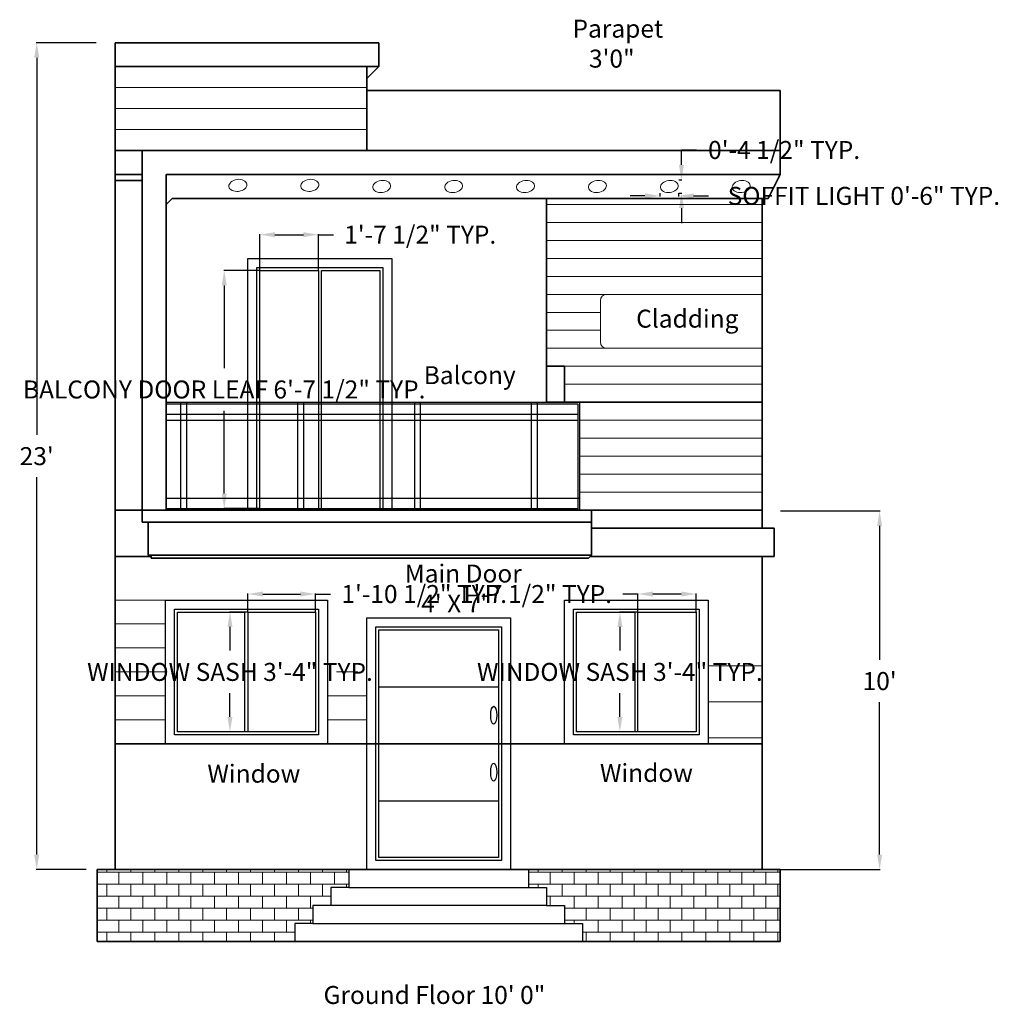
# Model space of a CAD drawing. Units: inches. Extents: x 103 to 430, y 16 to 345.
import ezdxf

# ---------------------------------------------------------------- set-up
doc = ezdxf.new("R2010")
doc.units = ezdxf.units.IN
doc.header["$MEASUREMENT"] = 0
for name, color, linetype, lineweight in [('A-ANNO-DIMS', 2, 'Continuous', 18), ('A-ANNO-TEXT', 7, 'Continuous', 25), ('A-DOOR', 4, 'Continuous', 25), ('A-ELEV', 7, 'Continuous', 35), ('A-ELEV-PATT', 8, 'Continuous', 13), ('A-FLOR-HRAL', 3, 'Continuous', 25), ('A-FLOR-STRS', 3, 'Continuous', 25), ('A-GLAZ', 4, 'Continuous', 25), ('E-LITE', 6, 'Continuous', 18)]:
    doc.layers.add(name, color=color, linetype=linetype, lineweight=lineweight)
doc.styles.get("Standard").update_dxf_attribs({"font": 'arial.ttf'})
doc.dimstyles.get("Standard").update_dxf_attribs({"dimtxt": 6, "dimasz": 5, "dimexe": 0.18, "dimexo": 0.0625, "dimgap": 4, "dimtad": 0, "dimtih": 1, "dimtoh": 1, "dimdec": 0, "dimzin": 0, "dimdsep": 46, "dimlunit": 3, "dimtxsty": 'Standard', "dimcen": 3, "dimadec": 0, "dimazin": 0, "dimtfac": 1, "dimtdec": 0, "dimtofl": 0, "dimtmove": 0, "dimatfit": 3, "dimfxl": 1, "dimtolj": 1, "dimtzin": 0, "dimarcsym": 0})

# ---------------------------------------------------------------- blocks, each defined once
blk = doc.blocks.new('*D1')
at = {"layer": 'A-ANNO-DIMS', "color": 0, "lineweight": -2, "transparency": 16777216}
for p, q in [((128.46, 336.91), (108.43, 336.91)), ((108.61, 331.91), (108.61, 205.97)), ((108.61, 65.91), (108.61, 191.84)), ((125.06, 60.91), (108.43, 60.91))]:
    blk.add_line(p, q, dxfattribs=at)
at = {"layer": 'A-ANNO-DIMS', "color": 0, "transparency": 16777216}
for points in [[(107.77, 331.91), (109.44, 331.91), (108.61, 336.91)], [(107.77, 65.91), (109.44, 65.91), (108.61, 60.91)]]:
    blk.add_solid(points, dxfattribs=at)
at = {"layer": 'Defpoints', "color": 0, "transparency": 16777216}
for p in [(128.53, 336.91), (108.61, 60.91), (125.12, 60.91)]:
    blk.add_point(p, dxfattribs=at)
at = {"layer": 'A-ANNO-DIMS', "color": 0, "transparency": 16777216, "insert": (108.61, 198.91), "char_height": 6, "attachment_point": 5}
blk.add_mtext("\\A1;23'", dxfattribs=at)
blk = doc.blocks.new('*D2')
at = {"layer": 'A-ANNO-DIMS', "color": 0, "lineweight": -2, "transparency": 16777216}
for p, q in [((356.83, 180.64), (390.15, 180.64)), ((389.97, 175.64), (389.97, 130.9)), ((389.97, 65.91), (389.97, 116.77)), ((356.83, 60.91), (390.15, 60.91))]:
    blk.add_line(p, q, dxfattribs=at)
at = {"layer": 'A-ANNO-DIMS', "color": 0, "transparency": 16777216}
for points in [[(389.14, 175.64), (390.8, 175.64), (389.97, 180.64)], [(389.14, 65.91), (390.8, 65.91), (389.97, 60.91)]]:
    blk.add_solid(points, dxfattribs=at)
at = {"layer": 'Defpoints', "color": 0, "transparency": 16777216}
for p in [(356.77, 180.64), (389.97, 180.64), (356.77, 60.91)]:
    blk.add_point(p, dxfattribs=at)
at = {"layer": 'A-ANNO-DIMS', "color": 0, "transparency": 16777216, "insert": (389.97, 123.84), "char_height": 6, "attachment_point": 5}
blk.add_mtext("\\A1;10'", dxfattribs=at)
blk = doc.blocks.new('DOOR-LEAF-BALC')
for p, q in [((0, 79.5), (19.5, 79.5)), ((0, 0), (0, 79.5)), ((19.5, 79.5), (19.5, 0))]:
    blk.add_line(p, q)
blk = doc.blocks.new('WIN-SASH-540')
blk.add_line((0, 40), (0, 0))
blk.add_lwpolyline([(0, 40), (22.5, 40), (22.5, 0), (0, 0)])
blk = doc.blocks.new('WIN-SASH-480')
blk.add_line((19.5, 40), (19.5, 0))
blk.add_lwpolyline([(19.5, 0), (0, 0), (0, 40), (19.5, 40)])
blk = doc.blocks.new('SOFFIT-LIGHT')
blk.add_ellipse((2.99, 2.02), major_axis=(2.98, 0.38), ratio=0.666667)
blk = doc.blocks.new('*D7')
at = {"layer": 'A-ANNO-DIMS', "color": 0, "lineweight": -2, "transparency": 16777216}
for p, q in [((316.65, 286.65), (316.65, 285.6)), ((322.88, 286.65), (322.88, 285.6)), ((311.65, 285.78), (306.65, 285.78)), ((327.88, 285.78), (332.88, 285.78))]:
    blk.add_line(p, q, dxfattribs=at)
at = {"layer": 'A-ANNO-DIMS', "color": 0, "transparency": 16777216}
for points in [[(311.65, 286.61), (311.65, 284.95), (316.65, 285.78)], [(327.88, 286.61), (327.88, 284.95), (322.88, 285.78)]]:
    blk.add_solid(points, dxfattribs=at)
at = {"layer": 'Defpoints', "color": 0, "transparency": 16777216}
for p in [(316.65, 286.71), (322.88, 286.71), (322.88, 285.78)]:
    blk.add_point(p, dxfattribs=at)
at = {"layer": 'A-ANNO-DIMS', "color": 0, "transparency": 16777216, "insert": (384.72, 285.78), "char_height": 6, "attachment_point": 5}
blk.add_mtext('\\A1;SOFFIT LIGHT 0\'-6" TYP.', dxfattribs=at)
blk = doc.blocks.new('*D8')
at = {"layer": 'A-ANNO-DIMS', "color": 0, "lineweight": -2, "transparency": 16777216}
for p, q in [((323.82, 296.1), (323.82, 301.1)), ((323.82, 301.1), (328.82, 301.1)), ((322.94, 291.1), (324, 291.1)), ((322.94, 286.71), (324, 286.71)), ((323.82, 281.71), (323.82, 276.71))]:
    blk.add_line(p, q, dxfattribs=at)
at = {"layer": 'A-ANNO-DIMS', "color": 0, "transparency": 16777216}
for points in [[(322.98, 296.1), (324.65, 296.1), (323.82, 291.1)], [(322.98, 281.71), (324.65, 281.71), (323.82, 286.71)]]:
    blk.add_solid(points, dxfattribs=at)
at = {"layer": 'Defpoints', "color": 0, "transparency": 16777216}
for p in [(322.88, 291.1), (323.82, 291.1), (322.88, 286.71)]:
    blk.add_point(p, dxfattribs=at)
at = {"layer": 'A-ANNO-DIMS', "color": 0, "transparency": 16777216, "insert": (358.09, 301.1), "char_height": 6, "attachment_point": 5}
blk.add_mtext('\\A1;0\'-4 1/2" TYP.', dxfattribs=at)
blk = doc.blocks.new('*D9')
at = {"layer": 'A-ANNO-DIMS', "color": 0, "lineweight": -2, "transparency": 16777216}
for p, q in [((183.06, 260.91), (171.02, 260.91)), ((171.2, 255.91), (171.2, 228.26)), ((171.2, 186.41), (171.2, 214.05)), ((183.06, 181.41), (171.02, 181.41))]:
    blk.add_line(p, q, dxfattribs=at)
at = {"layer": 'A-ANNO-DIMS', "color": 0, "transparency": 16777216}
for points in [[(170.36, 255.91), (172.03, 255.91), (171.2, 260.91)], [(170.36, 186.41), (172.03, 186.41), (171.2, 181.41)]]:
    blk.add_solid(points, dxfattribs=at)
at = {"layer": 'Defpoints', "color": 0, "transparency": 16777216}
for p in [(171.2, 260.91), (183.12, 260.91), (183.12, 181.41)]:
    blk.add_point(p, dxfattribs=at)
at = {"layer": 'A-ANNO-DIMS', "color": 0, "transparency": 16777216, "insert": (171.2, 221.16), "char_height": 6, "attachment_point": 5}
blk.add_mtext('\\A1;BALCONY DOOR LEAF 6\'-7 1/2" TYP.', dxfattribs=at)
blk = doc.blocks.new('*D10')
at = {"layer": 'A-ANNO-DIMS', "color": 0, "lineweight": -2, "transparency": 16777216}
for p, q in [((183.12, 260.97), (183.12, 273.01)), ((188.12, 272.83), (197.62, 272.83)), ((202.62, 260.97), (202.62, 273.01)), ((202.62, 272.83), (207.62, 272.83))]:
    blk.add_line(p, q, dxfattribs=at)
at = {"layer": 'A-ANNO-DIMS', "color": 0, "transparency": 16777216}
for points in [[(188.12, 273.66), (188.12, 272), (183.12, 272.83)], [(197.62, 273.66), (197.62, 272), (202.62, 272.83)]]:
    blk.add_solid(points, dxfattribs=at)
at = {"layer": 'Defpoints', "color": 0, "transparency": 16777216}
for p in [(202.62, 272.83), (183.12, 260.91), (202.62, 260.91)]:
    blk.add_point(p, dxfattribs=at)
at = {"layer": 'A-ANNO-DIMS', "color": 0, "transparency": 16777216, "insert": (236.62, 272.83), "char_height": 6, "attachment_point": 5}
blk.add_mtext('\\A1;1\'-7 1/2" TYP.', dxfattribs=at)
blk = doc.blocks.new('*D11')
at = {"layer": 'A-ANNO-DIMS', "color": 0, "lineweight": -2, "transparency": 16777216}
for p, q in [((179.06, 146.89), (172.94, 146.89)), ((173.12, 141.89), (173.12, 134)), ((173.12, 111.89), (173.12, 119.79)), ((179.06, 106.89), (172.94, 106.89))]:
    blk.add_line(p, q, dxfattribs=at)
at = {"layer": 'A-ANNO-DIMS', "color": 0, "transparency": 16777216}
for points in [[(172.29, 141.89), (173.96, 141.89), (173.12, 146.89)], [(172.29, 111.89), (173.96, 111.89), (173.12, 106.89)]]:
    blk.add_solid(points, dxfattribs=at)
at = {"layer": 'Defpoints', "color": 0, "transparency": 16777216}
for p in [(173.12, 146.89), (179.12, 146.89), (179.12, 106.89)]:
    blk.add_point(p, dxfattribs=at)
at = {"layer": 'A-ANNO-DIMS', "color": 0, "transparency": 16777216, "insert": (173.12, 126.89), "char_height": 6, "attachment_point": 5}
blk.add_mtext('\\A1;WINDOW SASH 3\'-4" TYP.', dxfattribs=at)
blk = doc.blocks.new('*D12')
at = {"layer": 'A-ANNO-DIMS', "color": 0, "lineweight": -2, "transparency": 16777216}
for p, q in [((179.12, 146.96), (179.12, 153.07)), ((184.12, 152.89), (196.62, 152.89)), ((201.62, 146.96), (201.62, 153.07)), ((201.62, 152.89), (206.62, 152.89))]:
    blk.add_line(p, q, dxfattribs=at)
at = {"layer": 'A-ANNO-DIMS', "color": 0, "transparency": 16777216}
for points in [[(184.12, 153.73), (184.12, 152.06), (179.12, 152.89)], [(196.62, 153.73), (196.62, 152.06), (201.62, 152.89)]]:
    blk.add_solid(points, dxfattribs=at)
at = {"layer": 'Defpoints', "color": 0, "transparency": 16777216}
for p in [(201.62, 152.89), (179.12, 146.89), (201.62, 146.89)]:
    blk.add_point(p, dxfattribs=at)
at = {"layer": 'A-ANNO-DIMS', "color": 0, "transparency": 16777216, "insert": (237.95, 152.89), "char_height": 6, "attachment_point": 5}
blk.add_mtext('\\A1;1\'-10 1/2" TYP.', dxfattribs=at)
blk = doc.blocks.new('*D13')
at = {"layer": 'A-ANNO-DIMS', "color": 0, "lineweight": -2, "transparency": 16777216}
for p, q in [((309.2, 146.89), (303.09, 146.89)), ((303.27, 141.89), (303.27, 134)), ((303.27, 111.89), (303.27, 119.79)), ((309.2, 106.89), (303.09, 106.89))]:
    blk.add_line(p, q, dxfattribs=at)
at = {"layer": 'A-ANNO-DIMS', "color": 0, "transparency": 16777216}
for points in [[(302.43, 141.89), (304.1, 141.89), (303.27, 146.89)], [(302.43, 111.89), (304.1, 111.89), (303.27, 106.89)]]:
    blk.add_solid(points, dxfattribs=at)
at = {"layer": 'Defpoints', "color": 0, "transparency": 16777216}
for p in [(309.27, 146.89), (303.27, 106.89), (309.27, 106.89)]:
    blk.add_point(p, dxfattribs=at)
at = {"layer": 'A-ANNO-DIMS', "color": 0, "transparency": 16777216, "insert": (303.27, 126.89), "char_height": 6, "attachment_point": 5}
blk.add_mtext('\\A1;WINDOW SASH 3\'-4" TYP.', dxfattribs=at)
blk = doc.blocks.new('*D14')
at = {"layer": 'A-ANNO-DIMS', "color": 0, "lineweight": -2, "transparency": 16777216}
for p, q in [((309.27, 152.89), (304.27, 152.89)), ((309.27, 146.96), (309.27, 153.07)), ((323.77, 152.89), (314.27, 152.89)), ((328.77, 146.96), (328.77, 153.07))]:
    blk.add_line(p, q, dxfattribs=at)
at = {"layer": 'A-ANNO-DIMS', "color": 0, "transparency": 16777216}
for points in [[(314.27, 153.73), (314.27, 152.06), (309.27, 152.89)], [(323.77, 153.73), (323.77, 152.06), (328.77, 152.89)]]:
    blk.add_solid(points, dxfattribs=at)
at = {"layer": 'Defpoints', "color": 0, "transparency": 16777216}
for p in [(309.27, 152.89), (309.27, 146.89), (328.77, 146.89)]:
    blk.add_point(p, dxfattribs=at)
at = {"layer": 'A-ANNO-DIMS', "color": 0, "transparency": 16777216, "insert": (275.27, 152.89), "char_height": 6, "attachment_point": 5}
blk.add_mtext('\\A1;1\'-7 1/2" TYP.', dxfattribs=at)

msp = doc.modelspace()

# ---------------------------------------------------------------- hatches: boundary and pattern name
at = {"layer": 'A-ELEV-PATT'}
h = msp.add_hatch(dxfattribs=at)
h.set_pattern_fill('AR-B816', color=256, scale=0.5)
h.paths.add_polyline_path([(206.77, 54.91), (212.77, 54.91), (212.77, 60.91), (134.77, 60.91), (128.77, 60.91), (128.77, 36.91), (134.77, 36.91), (194.77, 36.91), (194.77, 42.91), (200.77, 42.91), (200.77, 48.91), (206.77, 48.91)])
h.paths.add_polyline_path([(356.77, 60.91), (350.77, 60.91), (272.77, 60.91), (272.77, 54.91), (278.77, 54.91), (278.77, 48.91), (284.77, 48.91), (284.77, 42.91), (290.77, 42.91), (290.77, 36.91), (350.77, 36.91), (356.77, 36.91)])

# ---------------------------------------------------------------- linework, layer by layer
at = {"layer": 'A-DOOR'}
for p, q in [((179.12, 181.41), (179.12, 264.91)), ((179.12, 264.91), (227.12, 264.91)), ((227.12, 264.91), (227.12, 181.41)), ((182.12, 181.41), (182.12, 261.91)), ((182.12, 261.91), (224.12, 261.91)), ((224.12, 261.91), (224.12, 181.41)), ((222.77, 121.91), (262.77, 121.91)), ((222.77, 102.91), (262.77, 102.91)), ((222.77, 83.91), (262.77, 83.91))]:
    msp.add_line(p, q, dxfattribs=at)
for points in [[(218.77, 144.91), (266.77, 144.91), (266.77, 60.91), (218.77, 60.91)], [(221.77, 141.91), (263.77, 141.91), (263.77, 63.91), (221.77, 63.91)], [(222.77, 140.91), (262.77, 140.91), (262.77, 64.91), (222.77, 64.91)]]:
    msp.add_lwpolyline(points, close=True, dxfattribs=at)
for centre in [(261.17, 112.41), (261.17, 93.41)]:
    msp.add_ellipse(centre, major_axis=(0, 3), ratio=0.333333, dxfattribs=at)
at = {"layer": 'A-ELEV'}
for p, q in [((222.77, 336.91), (134.77, 336.91)), ((134.77, 336.91), (134.77, 60.91)), ((222.77, 328.91), (222.77, 336.91)), ((218.77, 328.91), (134.77, 328.91)), ((218.77, 320.91), (218.77, 328.91)), ((218.77, 328.91), (222.77, 328.91)), ((222.77, 328.91), (218.77, 324.91)), ((356.77, 320.91), (218.77, 320.91)), ((218.77, 320.91), (218.77, 300.91)), ((356.77, 300.91), (356.77, 320.91)), ((134.77, 300.91), (350.77, 300.91)), ((143.77, 180.91), (143.77, 300.91)), ((350.77, 300.91), (356.77, 300.91)), ((356.77, 300.91), (356.77, 292.91)), ((134.77, 292.91), (143.77, 292.91)), ((151.77, 180.91), (151.77, 292.91)), ((151.77, 292.91), (350.77, 292.91)), ((356.77, 292.91), (350.77, 292.91)), ((352.77, 284.91), (356.77, 292.91)), ((134.77, 290.91), (143.77, 290.91)), ((151.77, 282.91), (153.77, 284.91)), ((153.77, 284.91), (350.77, 284.91)), ((278.77, 284.91), (278.77, 216.91)), ((350.77, 284.91), (352.77, 284.91)), ((350.77, 174.91), (350.77, 284.91)), ((278.77, 228.91), (284.77, 228.91)), ((284.77, 228.91), (284.77, 216.91)), ((278.77, 216.91), (350.77, 216.91)), ((134.77, 180.91), (350.77, 180.91)), ((134.77, 180.91), (143.77, 180.91)), ((143.77, 180.91), (143.77, 176.91)), ((293.77, 176.91), (293.77, 180.91)), ((143.77, 176.91), (293.77, 176.91)), ((143.77, 176.91), (145.77, 176.91)), ((145.77, 176.91), (145.77, 165.91)), ((293.77, 165.91), (293.77, 176.91)), ((293.77, 174.91), (354.77, 174.91)), ((354.77, 174.91), (354.77, 165.41)), ((146.77, 165.41), (134.77, 165.41)), ((145.77, 165.91), (293.77, 165.91)), ((145.77, 165.91), (146.77, 165.91)), ((145.77, 165.91), (146.77, 165.91)), ((146.77, 165.91), (146.77, 164.91)), ((146.77, 164.91), (292.77, 164.91)), ((292.77, 164.91), (293.77, 165.91)), ((293.27, 165.41), (350.77, 165.41)), ((350.77, 60.91), (350.77, 165.41)), ((354.77, 165.41), (350.77, 165.41)), ((134.77, 102.89), (350.77, 102.89)), ((134.77, 60.91), (128.77, 60.91)), ((128.77, 60.91), (128.77, 36.91)), ((134.77, 60.91), (350.77, 60.91)), ((350.77, 60.91), (356.77, 60.91)), ((356.77, 60.91), (356.77, 36.91)), ((128.77, 36.91), (134.77, 36.91)), ((134.77, 36.91), (350.77, 36.91)), ((356.77, 36.91), (350.77, 36.91))]:
    msp.add_line(p, q, dxfattribs=at)
at = {"layer": 'A-ELEV-PATT'}
for p, q in [((218.77, 321.91), (134.77, 321.91)), ((218.77, 314.91), (134.77, 314.91)), ((218.77, 307.91), (134.77, 307.91)), ((278.77, 282.91), (350.77, 282.91)), ((278.77, 276.91), (350.77, 276.91)), ((278.77, 270.91), (350.77, 270.91)), ((278.77, 264.91), (350.77, 264.91)), ((278.77, 258.91), (350.77, 258.91)), ((278.77, 252.91), (350.77, 252.91)), ((296.77, 246.91), (296.77, 250.91)), ((298.77, 252.91), (332.77, 252.91)), ((350.77, 252.91), (350.77, 234.91)), ((278.77, 246.91), (296.77, 246.91)), ((296.77, 240.91), (296.77, 246.91)), ((278.77, 240.91), (296.77, 240.91)), ((296.77, 236.91), (296.77, 240.91)), ((278.77, 234.91), (350.77, 234.91)), ((332.77, 234.91), (298.77, 234.91)), ((278.77, 228.91), (350.77, 228.91)), ((284.77, 222.91), (350.77, 222.91)), ((289.77, 210.91), (350.77, 210.91)), ((289.77, 204.91), (350.77, 204.91)), ((289.77, 198.91), (350.77, 198.91)), ((289.77, 192.91), (350.77, 192.91)), ((289.77, 186.91), (350.77, 186.91)), ((151.62, 150.89), (134.77, 150.89)), ((151.62, 142.89), (134.77, 142.89)), ((151.62, 134.89), (134.77, 134.89)), ((332.77, 128.89), (350.77, 128.89)), ((151.62, 126.89), (134.77, 126.89)), ((208.63, 126.9), (215.77, 126.9)), ((151.62, 118.89), (134.77, 118.89)), ((205.61, 118.89), (218.75, 118.91)), ((332.77, 116.89), (350.77, 116.89)), ((151.62, 110.89), (134.77, 110.89)), ((205.62, 110.89), (218.76, 110.91)), ((205.62, 102.89), (218.77, 102.91)), ((332.77, 104.89), (350.77, 104.89)), ((332.77, 102.89), (350.77, 102.89))]:
    msp.add_line(p, q, dxfattribs=at)
for centre, start, end in [((298.77, 250.91), 90, 180), ((298.77, 236.91), 180, 270)]:
    msp.add_arc(centre, 2, start, end, dxfattribs=at)
at = {"layer": 'A-FLOR-HRAL'}
for p, q in [((151.77, 216.91), (289.77, 216.91)), ((156.77, 181.41), (156.77, 216.91)), ((158.77, 181.41), (158.77, 216.91)), ((195.77, 181.41), (195.77, 216.91)), ((197.77, 181.41), (197.77, 216.91)), ((234.77, 181.41), (234.77, 216.91)), ((236.77, 181.41), (236.77, 216.91)), ((273.77, 181.41), (273.77, 216.91)), ((275.77, 181.41), (275.77, 216.91)), ((289.77, 216.91), (289.77, 180.91)), ((151.77, 216.41), (289.27, 216.41)), ((289.27, 216.41), (289.27, 180.91)), ((151.77, 212.91), (289.27, 212.91)), ((151.77, 210.91), (289.27, 210.91)), ((151.77, 184.84), (289.62, 184.84)), ((151.77, 181.41), (289.27, 181.41))]:
    msp.add_line(p, q, dxfattribs=at)
at = {"layer": 'A-FLOR-STRS'}
for p, q in [((218.77, 60.91), (212.77, 60.91)), ((212.77, 60.91), (212.77, 54.91)), ((266.77, 60.91), (272.77, 60.91)), ((272.77, 60.91), (272.77, 54.91)), ((212.77, 54.91), (206.77, 54.91)), ((206.77, 54.91), (206.77, 48.91)), ((212.77, 54.91), (272.77, 54.91)), ((272.77, 54.91), (278.77, 54.91)), ((278.77, 54.91), (278.77, 48.91)), ((206.77, 48.91), (200.77, 48.91)), ((200.77, 48.91), (200.77, 42.91)), ((278.77, 48.91), (206.77, 48.91)), ((278.77, 48.91), (284.77, 48.91)), ((284.77, 48.91), (284.77, 42.91)), ((200.77, 42.91), (194.77, 42.91)), ((194.77, 42.91), (194.77, 36.91)), ((200.77, 42.91), (284.77, 42.91)), ((284.77, 42.91), (290.77, 42.91)), ((290.77, 42.91), (290.77, 36.91))]:
    msp.add_line(p, q, dxfattribs=at)
at = {"layer": 'A-GLAZ'}
for points in [[(205.62, 102.89), (151.62, 102.89), (151.62, 150.89), (205.62, 150.89)], [(202.62, 105.89), (154.62, 105.89), (154.62, 147.89), (202.62, 147.89)], [(332.77, 102.89), (284.77, 102.89), (284.77, 150.89), (332.77, 150.89)], [(329.77, 105.89), (287.77, 105.89), (287.77, 147.89), (329.77, 147.89)]]:
    msp.add_lwpolyline(points, close=True, dxfattribs=at)

# ---------------------------------------------------------------- block references
at = {"layer": 'A-DOOR'}
for p in [(183.12, 181.41), (203.62, 181.41)]:
    msp.add_blockref('DOOR-LEAF-BALC', p, dxfattribs=at)
at = {"layer": 'A-GLAZ', "rotation": 180}
for name, p in [('WIN-SASH-540', (178.12, 146.89)), ('WIN-SASH-480', (328.77, 146.89))]:
    msp.add_blockref(name, p, dxfattribs=at)
at = {"layer": 'A-GLAZ'}
for name, p in [('WIN-SASH-540', (179.12, 106.89)), ('WIN-SASH-480', (288.77, 106.89))]:
    msp.add_blockref(name, p, dxfattribs=at)
at = {"layer": 'E-LITE'}
for p in [(172.76, 287.26), (196.78, 287.26), (220.78, 286.89), (244.78, 286.89), (268.78, 286.89), (292.78, 286.89), (316.78, 286.89), (340.78, 286.89)]:
    msp.add_blockref('SOFFIT-LIGHT', p, dxfattribs=at)

# ---------------------------------------------------------------- texts
at = {"layer": 'A-ANNO-TEXT', "char_height": 6, "attachment_point": 1}
for s, width, insert in [('Parapet\\P   3\'0"', 50.7648, (287.46, 344.59)), ('Cladding', 50.7648, (308.7, 247.8)), ('Balcony', 50.7648, (237.79, 228.94)), ("Main Door\\P   4' X 7'", 50.7648, (231.46, 162.73)), ('Window', 50.7648, (165.57, 95.93)), ('Window', 50.7648, (296.61, 96.18)), ('Ground Floor 10\' 0"', 77.2992, (204.35, 22.06))]:
    msp.add_mtext_dynamic_manual_height_columns(s, width=width, gutter_width=1, heights=[0], dxfattribs=dict(at, insert=insert))

# ---------------------------------------------------------------- dimensions: what is measured, and where the dimension line sits
at = {"layer": 'A-ANNO-DIMS'}
dim = msp.add_linear_dim(base=(108.61, 60.91), p1=(128.53, 336.91), p2=(125.12, 60.91), angle=90, dimstyle='Standard', override={"dimclrd": 0, "dimclre": 0, "dimclrt": 0}, dxfattribs=at)
dim.commit()
dim.dimension.update_dxf_attribs({"geometry": '*D1', "text_midpoint": (108.61, 198.91)})
for base, p1, p2, angle, text, picture, middle in [((323.82, 291.1), (322.88, 286.71), (322.88, 291.1), 90, '<> TYP.', '*D8', (358.09, 301.1)), ((171.2, 260.91), (183.12, 181.41), (183.12, 260.91), 90, 'BALCONY DOOR LEAF <> TYP.', '*D9', (171.2, 221.16)), ((309.27, 152.89), (328.77, 146.89), (309.27, 146.89), 180, '<> TYP.', '*D14', (275.27, 152.89)), ((173.12, 146.89), (179.12, 106.89), (179.12, 146.89), 90, 'WINDOW SASH <> TYP.', '*D11', (173.12, 126.89)), ((303.27, 106.89), (309.27, 146.89), (309.27, 106.89), 270, 'WINDOW SASH <> TYP.', '*D13', (303.27, 126.89))]:
    dim = msp.add_linear_dim(base=base, p1=p1, p2=p2, angle=angle, text=text, dimstyle='Standard', override={"dimdec": 1, "dimrnd": 0, "dimzin": 1, "dimlunit": 4, "dimfrac": 2}, dxfattribs=at)
    dim.commit()
    dim.dimension.update_dxf_attribs({"geometry": picture, "text_midpoint": middle})
for base, p1, p2, text, picture, middle in [((322.88, 285.78), (316.65, 286.71), (322.88, 286.71), 'SOFFIT LIGHT <> TYP.', '*D7', (384.72, 285.78)), ((202.62, 272.83), (183.12, 260.91), (202.62, 260.91), '<> TYP.', '*D10', (236.62, 272.83)), ((201.62, 152.89), (179.12, 146.89), (201.62, 146.89), '<> TYP.', '*D12', (237.95, 152.89))]:
    dim = msp.add_linear_dim(base=base, p1=p1, p2=p2, text=text, dimstyle='Standard', override={"dimdec": 1, "dimrnd": 0, "dimzin": 1, "dimlunit": 4, "dimfrac": 2}, dxfattribs=at)
    dim.commit()
    dim.dimension.update_dxf_attribs({"geometry": picture, "text_midpoint": middle})
dim = msp.add_linear_dim(base=(389.97, 180.64), p1=(356.77, 60.91), p2=(356.77, 180.64), angle=90, dimstyle='Standard', override={"dimclrd": 0, "dimclre": 0, "dimclrt": 0}, dxfattribs=at)
dim.commit()
dim.dimension.update_dxf_attribs({"geometry": '*D2', "text_midpoint": (389.97, 123.84), "dimtype": 160})

doc.saveas('drawing.dxf')
